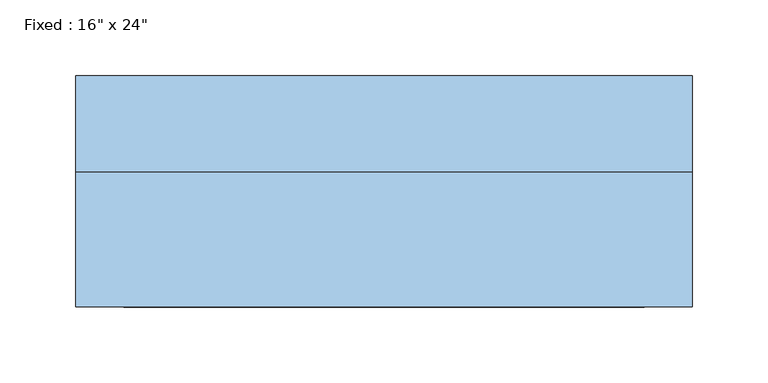
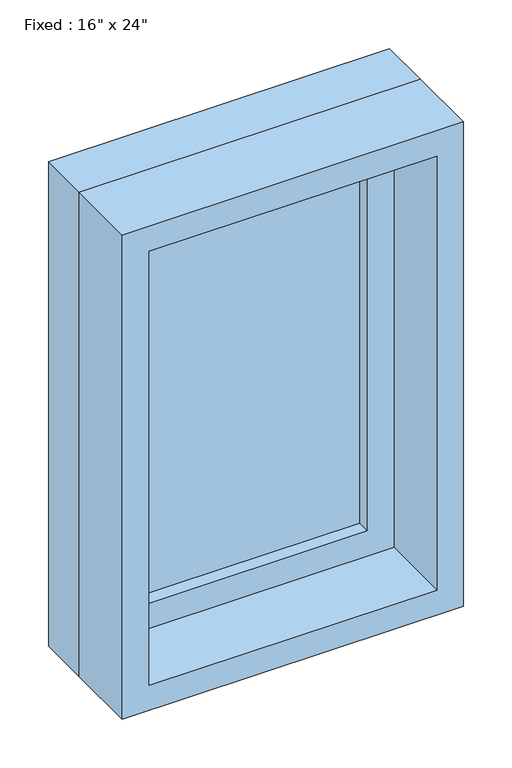
"""IFC4 building model written with IfcOpenShell, lengths in millimetres: window geometry."""

from ifc_helpers import new_model, si_unit, frame, origin, place, context, project, spatial, polyline, outline, extrude, source, transform, mapped, element, save


def window_7ecdf1d7(model_context):
    return source(origin(), model_context, "Body", "SweptSolid", [
        extrude(outline(polyline([(101.6, 28.575), (-177.8, 28.575), (-177.8, 41.275), (101.6, 41.275), (101.6, 28.575)])), frame((0.0, 0.0, 977.9), z_axis=(0.0, 0.0, 1.0), x_axis=(1.0, 0.0, 0.0)), (0.0, 0.0, 1.0), 482.6),
        extrude(outline(polyline([(1504.95, -222.25), (933.45, -222.25), (933.45, 146.05), (1504.95, 146.05), (1504.95, -222.25)]), holes=[polyline([(1460.5, -177.8), (1460.5, 101.6), (977.9, 101.6), (977.9, -177.8), (1460.5, -177.8)])]), frame((0.0, 12.7, 0.0), z_axis=(0.0, 1.0, 0.0), x_axis=(0.0, 0.0, 1.0)), (0.0, 0.0, 1.0), 44.45),
        extrude(outline(polyline([(1524.0, -241.3), (914.4, -241.3), (914.4, 165.1), (1524.0, 165.1), (1524.0, -241.3)]), holes=[polyline([(1492.25, -209.55), (1492.25, 133.35), (946.15, 133.35), (946.15, -209.55), (1492.25, -209.55)])]), frame((0.0, -76.2, 0.0), z_axis=(0.0, 1.0, 0.0), x_axis=(0.0, 0.0, 1.0)), (0.0, 0.0, 1.0), 88.9),
        extrude(outline(polyline([(1524.0, 165.1), (1524.0, -241.3), (914.4, -241.3), (914.4, 165.1), (1524.0, 165.1)]), holes=[polyline([(1504.95, 146.05), (933.45, 146.05), (933.45, -222.25), (1504.95, -222.25), (1504.95, 146.05)])]), frame((0.0, 12.7, 0.0), z_axis=(0.0, 1.0, 0.0), x_axis=(0.0, 0.0, 1.0)), (0.0, 0.0, 1.0), 63.5),
    ])


if __name__ == "__main__":
    model = new_model("IFC4")
    model_context = context("Model", 3, world=origin())
    ifc_project = project(units=[si_unit("LENGTHUNIT", "METRE", prefix="MILLI")], contexts=[model_context])
    site = spatial("IfcSite", under=ifc_project)
    building = spatial("IfcBuilding", under=site)
    placement = place(None, origin())
    window_shape = window_7ecdf1d7(model_context)
    element("IfcWindow", 1, ObjectType="Fixed : 16\" x 24\"", at=placement, inside=building, context=model_context, shape_type="MappedRepresentation", body=[
        mapped(window_shape, transform((0.0, 0.0, 0.0), x_axis=(1.0, 0.0, 0.0), y_axis=(0.0, 1.0, 0.0), z_axis=(0.0, 0.0, 1.0))),
    ])
    save(model, "model.ifc")

# Revit data of these elements
# Type "Fixed : 16\" x 24\""
#   Type Mark = "4"
#   Construction Type Id = "GSP4R"
#   Assembly Code = "B2020100"
#   Analytic Construction = "1/8 in Pilkington single glazing"
#   Visual Light Transmittance = 0.9
#   Solar Heat Gain Coefficient = 0.78
#   Heat Transfer Coefficient (U) = 0.6496 BTU/(h·ft²·°F)
#   Height = 2' - 0"
#   Default Sill Height = 3' - 0"
#   Width = 1' - 4"
#   Window Inset = 0' - 0 3/4"
#   Define Thermal Properties by = 1
#   Glass Pane Material = Glass
#   Sash Material = Sash
#   Wall Closure = (empty or 0)
# Element 1 (IfcWindow, "Fixed : 16\" x 24\"")
#   Materials on its faces: "Sash", "Glass"
# Materials
#   "Glass": class "Glass", colour RGB 0 128 192, transparency 0.75, Description = "Soda Lime Glass", Cost = 0
#   "Sash": class "Wood", colour RGB 224 178 126, transparency 0
